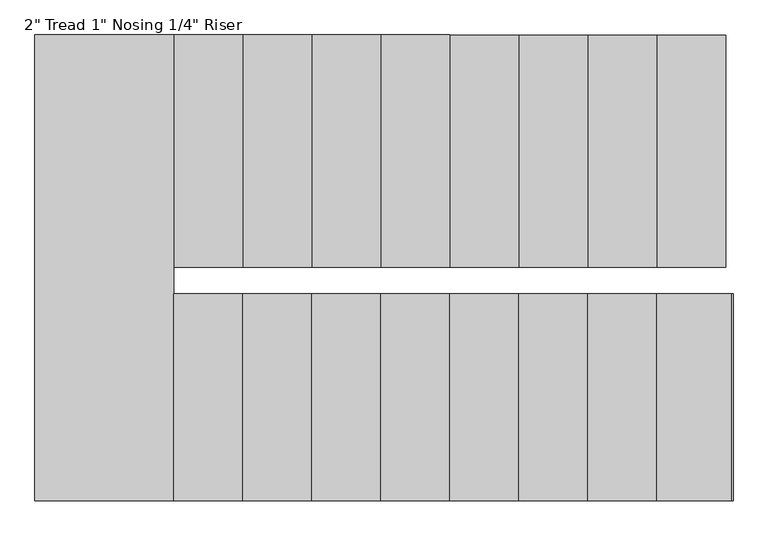
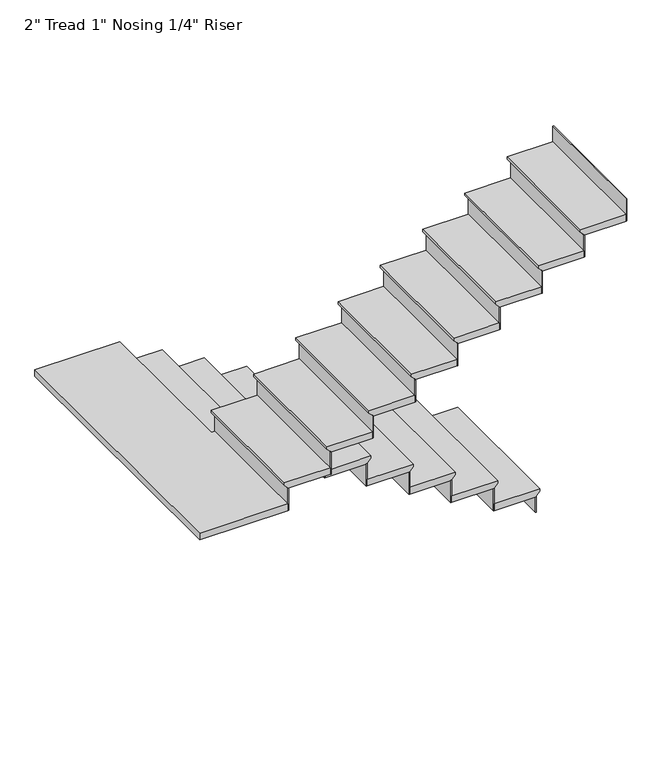
"""IFC4 building model written with IfcOpenShell, lengths in millimetres: stair flight geometry."""

from ifc_helpers import new_model, si_unit, origin, place, context, project, spatial, faceted_brep, source, transform, mapped, element, save


def stair_flight_289fc41f(model_context):
    return source(origin(), model_context, "Body", "Brep", [
        faceted_brep([(4295.1355783, 9969.5, 3198.2833333), (4295.1355783, 9969.5, 3217.3333333), (4295.1355783, 8944.6068332, 3217.3333333), (4295.1355783, 8944.6068332, 3198.2833333), (4269.7355783, 9969.5, 3172.8833333), (4269.7355783, 8944.6068332, 3172.8833333), (3964.9355783, 9969.5, 3217.3333333), (3964.9355783, 8944.6068332, 3217.3333333), (4269.7355783, 8944.6068332, 3166.5333333), (3964.9355783, 8944.6068332, 3166.5333333), (3964.9355783, 9969.5, 3166.5333333), (4269.7355783, 9969.5, 3166.5333333)], [[[0, 1, 2, 3]], [[4, 0, 3, 5]], [[2, 1, 6, 7]], [[8, 9, 10, 11]], [[2, 7, 9, 8, 5, 3]], [[8, 11, 4, 5]], [[6, 1, 0, 4, 11, 10]], [[7, 6, 10, 9]]]),
        faceted_brep([(4269.7355783, 9969.5, 3166.5333333), (4269.7355783, 9969.5, 3048.0), (4263.3855783, 9969.5, 3048.0), (4263.3855783, 9969.5, 3166.5333333), (4269.7355783, 8944.6068332, 3166.5333333), (4263.3855783, 8944.6068332, 3166.5333333), (4263.3855783, 8944.6068332, 3048.0), (4269.7355783, 8944.6068332, 3048.0)], [[[0, 1, 2, 3]], [[4, 5, 6, 7]], [[1, 0, 4, 7]], [[2, 1, 7, 6]], [[3, 2, 6, 5]], [[0, 3, 5, 4]]]),
        faceted_brep([(3964.9355783, 9969.5, 3335.8666667), (3964.9355783, 9969.5, 3166.5333333), (3958.5855783, 9969.5, 3166.5333333), (3958.5855783, 9969.5, 3335.8666667), (3964.9355783, 8944.6068332, 3335.8666667), (3958.5855783, 8944.6068332, 3335.8666667), (3958.5855783, 8944.6068332, 3166.5333333), (3964.9355783, 8944.6068332, 3166.5333333)], [[[0, 1, 2, 3]], [[4, 5, 6, 7]], [[1, 0, 4, 7]], [[2, 1, 7, 6]], [[3, 2, 6, 5]], [[0, 3, 5, 4]]]),
        faceted_brep([(3990.3355783, 8944.6068332, 3386.6666667), (3990.3355783, 9969.5, 3386.6666667), (3660.1355783, 9969.5, 3386.6666667), (3660.1355783, 8944.6068332, 3386.6666667), (3964.9355783, 8944.6068332, 3335.8666667), (3660.1355783, 8944.6068332, 3335.8666667), (3660.1355783, 9969.5, 3335.8666667), (3964.9355783, 9969.5, 3335.8666667), (3964.9355783, 8944.6068332, 3342.2166667), (3990.3355783, 8944.6068332, 3367.6166667), (3964.9355783, 9969.5, 3342.2166667), (3990.3355783, 9969.5, 3367.6166667)], [[[0, 1, 2, 3]], [[4, 5, 6, 7]], [[0, 3, 5, 4, 8, 9]], [[4, 7, 10, 8]], [[2, 1, 11, 10, 7, 6]], [[3, 2, 6, 5]], [[11, 1, 0, 9]], [[10, 11, 9, 8]]]),
        faceted_brep([(3660.1355783, 9969.5, 3505.2), (3660.1355783, 9969.5, 3335.8666667), (3653.7855783, 9969.5, 3335.8666667), (3653.7855783, 9969.5, 3505.2), (3660.1355783, 8944.6068332, 3505.2), (3653.7855783, 8944.6068332, 3505.2), (3653.7855783, 8944.6068332, 3335.8666667), (3660.1355783, 8944.6068332, 3335.8666667)], [[[0, 1, 2, 3]], [[4, 5, 6, 7]], [[1, 0, 4, 7]], [[2, 1, 7, 6]], [[3, 2, 6, 5]], [[0, 3, 5, 4]]]),
        faceted_brep([(3685.5355783, 8944.6068332, 3556.0), (3685.5355783, 9969.5, 3556.0), (3355.3355783, 9969.5, 3556.0), (3355.3355783, 8944.6068332, 3556.0), (3660.1355783, 8944.6068332, 3505.2), (3355.3355783, 8944.6068332, 3505.2), (3355.3355783, 9969.5, 3505.2), (3660.1355783, 9969.5, 3505.2), (3660.1355783, 8944.6068332, 3511.55), (3685.5355783, 8944.6068332, 3536.95), (3660.1355783, 9969.5, 3511.55), (3685.5355783, 9969.5, 3536.95)], [[[0, 1, 2, 3]], [[4, 5, 6, 7]], [[0, 3, 5, 4, 8, 9]], [[4, 7, 10, 8]], [[2, 1, 11, 10, 7, 6]], [[3, 2, 6, 5]], [[11, 1, 0, 9]], [[10, 11, 9, 8]]]),
        faceted_brep([(3355.3355783, 9969.5, 3674.5333333), (3355.3355783, 9969.5, 3505.2), (3348.9855783, 9969.5, 3505.2), (3348.9855783, 9969.5, 3674.5333333), (3355.3355783, 8944.6068332, 3674.5333333), (3348.9855783, 8944.6068332, 3674.5333333), (3348.9855783, 8944.6068332, 3505.2), (3355.3355783, 8944.6068332, 3505.2)], [[[0, 1, 2, 3]], [[4, 5, 6, 7]], [[1, 0, 4, 7]], [[2, 1, 7, 6]], [[3, 2, 6, 5]], [[0, 3, 5, 4]]]),
        faceted_brep([(3380.7355783, 8944.6068332, 3725.3333333), (3380.7355783, 9969.5, 3725.3333333), (3050.5355783, 9969.5, 3725.3333333), (3050.5355783, 8944.6068332, 3725.3333333), (3355.3355783, 8944.6068332, 3674.5333333), (3050.5355783, 8944.6068332, 3674.5333333), (3050.5355783, 9969.5, 3674.5333333), (3355.3355783, 9969.5, 3674.5333333), (3355.3355783, 8944.6068332, 3680.8833333), (3380.7355783, 8944.6068332, 3706.2833333), (3355.3355783, 9969.5, 3680.8833333), (3380.7355783, 9969.5, 3706.2833333)], [[[0, 1, 2, 3]], [[4, 5, 6, 7]], [[0, 3, 5, 4, 8, 9]], [[4, 7, 10, 8]], [[2, 1, 11, 10, 7, 6]], [[3, 2, 6, 5]], [[11, 1, 0, 9]], [[10, 11, 9, 8]]]),
        faceted_brep([(3050.5355783, 9969.5, 3843.8666667), (3050.5355783, 9969.5, 3674.5333333), (3044.1855783, 9969.5, 3674.5333333), (3044.1855783, 9969.5, 3843.8666667), (3050.5355783, 8944.6068332, 3843.8666667), (3044.1855783, 8944.6068332, 3843.8666667), (3044.1855783, 8944.6068332, 3674.5333333), (3050.5355783, 8944.6068332, 3674.5333333)], [[[0, 1, 2, 3]], [[4, 5, 6, 7]], [[1, 0, 4, 7]], [[2, 1, 7, 6]], [[3, 2, 6, 5]], [[0, 3, 5, 4]]]),
        faceted_brep([(3075.9355783, 8944.6068332, 3894.6666667), (3075.9355783, 9969.5, 3894.6666667), (2745.7355783, 9969.5, 3894.6666667), (2745.7355783, 8944.6068332, 3894.6666667), (3050.5355783, 8944.6068332, 3843.8666667), (2745.7355783, 8944.6068332, 3843.8666667), (2745.7355783, 9969.5, 3843.8666667), (3050.5355783, 9969.5, 3843.8666667), (3050.5355783, 8944.6068332, 3850.2166667), (3075.9355783, 8944.6068332, 3875.6166667), (3050.5355783, 9969.5, 3850.2166667), (3075.9355783, 9969.5, 3875.6166667)], [[[0, 1, 2, 3]], [[4, 5, 6, 7]], [[0, 3, 5, 4, 8, 9]], [[4, 7, 10, 8]], [[2, 1, 11, 10, 7, 6]], [[3, 2, 6, 5]], [[11, 1, 0, 9]], [[10, 11, 9, 8]]]),
        faceted_brep([(2745.7355783, 9969.5, 4013.2), (2745.7355783, 9969.5, 3843.8666667), (2739.3855783, 9969.5, 3843.8666667), (2739.3855783, 9969.5, 4013.2), (2745.7355783, 8944.6068332, 4013.2), (2739.3855783, 8944.6068332, 4013.2), (2739.3855783, 8944.6068332, 3843.8666667), (2745.7355783, 8944.6068332, 3843.8666667)], [[[0, 1, 2, 3]], [[4, 5, 6, 7]], [[1, 0, 4, 7]], [[2, 1, 7, 6]], [[3, 2, 6, 5]], [[0, 3, 5, 4]]]),
        faceted_brep([(2771.1355783, 8944.6068332, 4064.0), (2771.1355783, 9969.5, 4064.0), (2440.9355783, 9969.5, 4064.0), (2440.9355783, 8944.6068332, 4064.0), (2745.7355783, 8944.6068332, 4013.2), (2440.9355783, 8944.6068332, 4013.2), (2440.9355783, 9969.5, 4013.2), (2745.7355783, 9969.5, 4013.2), (2745.7355783, 8944.6068332, 4019.55), (2771.1355783, 8944.6068332, 4044.95), (2745.7355783, 9969.5, 4019.55), (2771.1355783, 9969.5, 4044.95)], [[[0, 1, 2, 3]], [[4, 5, 6, 7]], [[0, 3, 5, 4, 8, 9]], [[4, 7, 10, 8]], [[2, 1, 11, 10, 7, 6]], [[3, 2, 6, 5]], [[11, 1, 0, 9]], [[10, 11, 9, 8]]]),
        faceted_brep([(2440.9355783, 9969.5, 4182.5333333), (2440.9355783, 9969.5, 4013.2), (2434.5855783, 9969.5, 4013.2), (2434.5855783, 9969.5, 4182.5333333), (2440.9355783, 8944.6068332, 4182.5333333), (2434.5855783, 8944.6068332, 4182.5333333), (2434.5855783, 8944.6068332, 4013.2), (2440.9355783, 8944.6068332, 4013.2)], [[[0, 1, 2, 3]], [[4, 5, 6, 7]], [[1, 0, 4, 7]], [[2, 1, 7, 6]], [[3, 2, 6, 5]], [[0, 3, 5, 4]]]),
        faceted_brep([(2466.3355783, 8944.6068332, 4233.3333333), (2466.3355783, 9969.5, 4233.3333333), (2136.1355783, 9969.5, 4233.3333333), (2136.1355783, 8944.6068332, 4233.3333333), (2440.9355783, 8944.6068332, 4182.5333333), (2136.1355783, 8944.6068332, 4182.5333333), (2136.1355783, 9969.5, 4182.5333333), (2440.9355783, 9969.5, 4182.5333333), (2440.9355783, 8944.6068332, 4188.8833333), (2466.3355783, 8944.6068332, 4214.2833333), (2440.9355783, 9969.5, 4188.8833333), (2466.3355783, 9969.5, 4214.2833333)], [[[0, 1, 2, 3]], [[4, 5, 6, 7]], [[0, 3, 5, 4, 8, 9]], [[4, 7, 10, 8]], [[2, 1, 11, 10, 7, 6]], [[3, 2, 6, 5]], [[11, 1, 0, 9]], [[10, 11, 9, 8]]]),
        faceted_brep([(2136.1355783, 9969.5, 4351.8666667), (2136.1355783, 9969.5, 4182.5333333), (2129.7855783, 9969.5, 4182.5333333), (2129.7855783, 9969.5, 4351.8666667), (2136.1355783, 8944.6068332, 4351.8666667), (2129.7855783, 8944.6068332, 4351.8666667), (2129.7855783, 8944.6068332, 4182.5333333), (2136.1355783, 8944.6068332, 4182.5333333)], [[[0, 1, 2, 3]], [[4, 5, 6, 7]], [[1, 0, 4, 7]], [[2, 1, 7, 6]], [[3, 2, 6, 5]], [[0, 3, 5, 4]]]),
        faceted_brep([(2161.5355783, 8944.6068332, 4402.6666667), (2161.5355783, 9969.5, 4402.6666667), (1831.3355783, 9969.5, 4402.6666667), (1831.3355783, 8944.6068332, 4402.6666667), (2136.1355783, 8944.6068332, 4351.8666667), (1831.3355783, 8944.6068332, 4351.8666667), (1831.3355783, 9969.5, 4351.8666667), (2136.1355783, 9969.5, 4351.8666667), (2136.1355783, 8944.6068332, 4358.2166667), (2161.5355783, 8944.6068332, 4383.6166667), (2136.1355783, 9969.5, 4358.2166667), (2161.5355783, 9969.5, 4383.6166667)], [[[0, 1, 2, 3]], [[4, 5, 6, 7]], [[0, 3, 5, 4, 8, 9]], [[4, 7, 10, 8]], [[2, 1, 11, 10, 7, 6]], [[3, 2, 6, 5]], [[11, 1, 0, 9]], [[10, 11, 9, 8]]]),
        faceted_brep([(1831.3355783, 9969.5, 4521.2), (1831.3355783, 9969.5, 4351.8666667), (1824.9855783, 9969.5, 4351.8666667), (1824.9855783, 9969.5, 4521.2), (1831.3355783, 8944.6068332, 4521.2), (1824.9855783, 8944.6068332, 4521.2), (1824.9855783, 8944.6068332, 4351.8666667), (1831.3355783, 8944.6068332, 4351.8666667)], [[[0, 1, 2, 3]], [[4, 5, 6, 7]], [[1, 0, 4, 7]], [[2, 1, 7, 6]], [[3, 2, 6, 5]], [[0, 3, 5, 4]]]),
        faceted_brep([(1882.1355783, 8826.5, 4572.0), (1856.7355783, 8826.5, 4572.0), (1856.7355783, 9969.5, 4572.0), (1244.6, 9969.5, 4572.0), (1244.6, 7912.1, 4572.0), (1882.1355783, 7912.1, 4572.0), (1856.7355783, 8826.5, 4521.2), (1882.1355783, 8826.5, 4521.2), (1882.1355783, 7912.1, 4521.2), (1244.6, 7912.1, 4521.2), (1244.6, 9969.5, 4521.2), (1831.3355783, 9969.5, 4521.2), (1831.3355783, 8944.6068332, 4521.2), (1856.7355783, 8944.6068332, 4521.2), (1856.7355783, 8944.6068332, 4552.95), (1856.7355783, 9969.5, 4552.95), (1831.3355783, 8944.6068332, 4527.55), (1831.3355783, 9969.5, 4527.55)], [[[0, 1, 2, 3, 4, 5]], [[6, 7, 8, 9, 10, 11, 12, 13]], [[1, 0, 7, 6]], [[2, 1, 6, 13, 14, 15]], [[13, 12, 16, 14]], [[12, 11, 17, 16]], [[3, 2, 15, 17, 11, 10]], [[4, 3, 10, 9]], [[5, 4, 9, 8]], [[0, 5, 8, 7]], [[17, 15, 14, 16]]]),
        faceted_brep([(1882.1355783, 7912.1, 4690.5333333), (1882.1355783, 7912.1, 4521.2), (1888.4855783, 7912.1, 4521.2), (1888.4855783, 7912.1, 4690.5333333), (1882.1355783, 8826.5, 4690.5333333), (1888.4855783, 8826.5, 4690.5333333), (1888.4855783, 8826.5, 4521.2), (1882.1355783, 8826.5, 4521.2)], [[[0, 1, 2, 3]], [[4, 5, 6, 7]], [[1, 0, 4, 7]], [[2, 1, 7, 6]], [[3, 2, 6, 5]], [[0, 3, 5, 4]]]),
        faceted_brep([(1856.7355783, 8826.5, 4741.3333333), (1856.7355783, 7912.1, 4741.3333333), (2186.9355783, 7912.1, 4741.3333333), (2186.9355783, 8826.5, 4741.3333333), (1882.1355783, 8826.5, 4690.5333333), (2186.9355783, 8826.5, 4690.5333333), (2186.9355783, 7912.1, 4690.5333333), (1882.1355783, 7912.1, 4690.5333333), (1882.1355783, 8826.5, 4696.8833333), (1856.7355783, 8826.5, 4722.2833333), (1882.1355783, 7912.1, 4696.8833333), (1856.7355783, 7912.1, 4722.2833333)], [[[0, 1, 2, 3]], [[4, 5, 6, 7]], [[0, 3, 5, 4, 8, 9]], [[4, 7, 10, 8]], [[2, 1, 11, 10, 7, 6]], [[3, 2, 6, 5]], [[11, 1, 0, 9]], [[10, 11, 9, 8]]]),
        faceted_brep([(2186.9355783, 7912.1, 4859.8666667), (2186.9355783, 7912.1, 4690.5333333), (2193.2855783, 7912.1, 4690.5333333), (2193.2855783, 7912.1, 4859.8666667), (2186.9355783, 8826.5, 4859.8666667), (2193.2855783, 8826.5, 4859.8666667), (2193.2855783, 8826.5, 4690.5333333), (2186.9355783, 8826.5, 4690.5333333)], [[[0, 1, 2, 3]], [[4, 5, 6, 7]], [[1, 0, 4, 7]], [[2, 1, 7, 6]], [[3, 2, 6, 5]], [[0, 3, 5, 4]]]),
        faceted_brep([(2161.5355783, 8826.5, 4910.6666667), (2161.5355783, 7912.1, 4910.6666667), (2491.7355783, 7912.1, 4910.6666667), (2491.7355783, 8826.5, 4910.6666667), (2186.9355783, 8826.5, 4859.8666667), (2491.7355783, 8826.5, 4859.8666667), (2491.7355783, 7912.1, 4859.8666667), (2186.9355783, 7912.1, 4859.8666667), (2186.9355783, 8826.5, 4866.2166667), (2161.5355783, 8826.5, 4891.6166667), (2186.9355783, 7912.1, 4866.2166667), (2161.5355783, 7912.1, 4891.6166667)], [[[0, 1, 2, 3]], [[4, 5, 6, 7]], [[0, 3, 5, 4, 8, 9]], [[4, 7, 10, 8]], [[2, 1, 11, 10, 7, 6]], [[3, 2, 6, 5]], [[11, 1, 0, 9]], [[10, 11, 9, 8]]]),
        faceted_brep([(2491.7355783, 7912.1, 5029.2), (2491.7355783, 7912.1, 4859.8666667), (2498.0855783, 7912.1, 4859.8666667), (2498.0855783, 7912.1, 5029.2), (2491.7355783, 8826.5, 5029.2), (2498.0855783, 8826.5, 5029.2), (2498.0855783, 8826.5, 4859.8666667), (2491.7355783, 8826.5, 4859.8666667)], [[[0, 1, 2, 3]], [[4, 5, 6, 7]], [[1, 0, 4, 7]], [[2, 1, 7, 6]], [[3, 2, 6, 5]], [[0, 3, 5, 4]]]),
        faceted_brep([(2466.3355783, 8826.5, 5080.0), (2466.3355783, 7912.1, 5080.0), (2796.5355783, 7912.1, 5080.0), (2796.5355783, 8826.5, 5080.0), (2491.7355783, 8826.5, 5029.2), (2796.5355783, 8826.5, 5029.2), (2796.5355783, 7912.1, 5029.2), (2491.7355783, 7912.1, 5029.2), (2491.7355783, 8826.5, 5035.55), (2466.3355783, 8826.5, 5060.95), (2491.7355783, 7912.1, 5035.55), (2466.3355783, 7912.1, 5060.95)], [[[0, 1, 2, 3]], [[4, 5, 6, 7]], [[0, 3, 5, 4, 8, 9]], [[4, 7, 10, 8]], [[2, 1, 11, 10, 7, 6]], [[3, 2, 6, 5]], [[11, 1, 0, 9]], [[10, 11, 9, 8]]]),
        faceted_brep([(2796.5355783, 7912.1, 5198.5333333), (2796.5355783, 7912.1, 5029.2), (2802.8855783, 7912.1, 5029.2), (2802.8855783, 7912.1, 5198.5333333), (2796.5355783, 8826.5, 5198.5333333), (2802.8855783, 8826.5, 5198.5333333), (2802.8855783, 8826.5, 5029.2), (2796.5355783, 8826.5, 5029.2)], [[[0, 1, 2, 3]], [[4, 5, 6, 7]], [[1, 0, 4, 7]], [[2, 1, 7, 6]], [[3, 2, 6, 5]], [[0, 3, 5, 4]]]),
        faceted_brep([(2771.1355783, 8826.5, 5249.3333333), (2771.1355783, 7912.1, 5249.3333333), (3101.3355783, 7912.1, 5249.3333333), (3101.3355783, 8826.5, 5249.3333333), (2796.5355783, 8826.5, 5198.5333333), (3101.3355783, 8826.5, 5198.5333333), (3101.3355783, 7912.1, 5198.5333333), (2796.5355783, 7912.1, 5198.5333333), (2796.5355783, 8826.5, 5204.8833333), (2771.1355783, 8826.5, 5230.2833333), (2796.5355783, 7912.1, 5204.8833333), (2771.1355783, 7912.1, 5230.2833333)], [[[0, 1, 2, 3]], [[4, 5, 6, 7]], [[0, 3, 5, 4, 8, 9]], [[4, 7, 10, 8]], [[2, 1, 11, 10, 7, 6]], [[3, 2, 6, 5]], [[11, 1, 0, 9]], [[10, 11, 9, 8]]]),
        faceted_brep([(3101.3355783, 7912.1, 5367.8666667), (3101.3355783, 7912.1, 5198.5333333), (3107.6855783, 7912.1, 5198.5333333), (3107.6855783, 7912.1, 5367.8666667), (3101.3355783, 8826.5, 5367.8666667), (3107.6855783, 8826.5, 5367.8666667), (3107.6855783, 8826.5, 5198.5333333), (3101.3355783, 8826.5, 5198.5333333)], [[[0, 1, 2, 3]], [[4, 5, 6, 7]], [[1, 0, 4, 7]], [[2, 1, 7, 6]], [[3, 2, 6, 5]], [[0, 3, 5, 4]]]),
        faceted_brep([(3075.9355783, 8826.5, 5418.6666667), (3075.9355783, 7912.1, 5418.6666667), (3406.1355783, 7912.1, 5418.6666667), (3406.1355783, 8826.5, 5418.6666667), (3101.3355783, 8826.5, 5367.8666667), (3406.1355783, 8826.5, 5367.8666667), (3406.1355783, 7912.1, 5367.8666667), (3101.3355783, 7912.1, 5367.8666667), (3101.3355783, 8826.5, 5374.2166667), (3075.9355783, 8826.5, 5399.6166667), (3101.3355783, 7912.1, 5374.2166667), (3075.9355783, 7912.1, 5399.6166667)], [[[0, 1, 2, 3]], [[4, 5, 6, 7]], [[0, 3, 5, 4, 8, 9]], [[4, 7, 10, 8]], [[2, 1, 11, 10, 7, 6]], [[3, 2, 6, 5]], [[11, 1, 0, 9]], [[10, 11, 9, 8]]]),
        faceted_brep([(3406.1355783, 7912.1, 5537.2), (3406.1355783, 7912.1, 5367.8666667), (3412.4855783, 7912.1, 5367.8666667), (3412.4855783, 7912.1, 5537.2), (3406.1355783, 8826.5, 5537.2), (3412.4855783, 8826.5, 5537.2), (3412.4855783, 8826.5, 5367.8666667), (3406.1355783, 8826.5, 5367.8666667)], [[[0, 1, 2, 3]], [[4, 5, 6, 7]], [[1, 0, 4, 7]], [[2, 1, 7, 6]], [[3, 2, 6, 5]], [[0, 3, 5, 4]]]),
        faceted_brep([(3380.7355783, 8826.5, 5588.0), (3380.7355783, 7912.1, 5588.0), (3710.9355783, 7912.1, 5588.0), (3710.9355783, 8826.5, 5588.0), (3406.1355783, 8826.5, 5537.2), (3710.9355783, 8826.5, 5537.2), (3710.9355783, 7912.1, 5537.2), (3406.1355783, 7912.1, 5537.2), (3406.1355783, 8826.5, 5543.55), (3380.7355783, 8826.5, 5568.95), (3406.1355783, 7912.1, 5543.55), (3380.7355783, 7912.1, 5568.95)], [[[0, 1, 2, 3]], [[4, 5, 6, 7]], [[0, 3, 5, 4, 8, 9]], [[4, 7, 10, 8]], [[2, 1, 11, 10, 7, 6]], [[3, 2, 6, 5]], [[11, 1, 0, 9]], [[10, 11, 9, 8]]]),
        faceted_brep([(3710.9355783, 7912.1, 5706.5333333), (3710.9355783, 7912.1, 5537.2), (3717.2855783, 7912.1, 5537.2), (3717.2855783, 7912.1, 5706.5333333), (3710.9355783, 8826.5, 5706.5333333), (3717.2855783, 8826.5, 5706.5333333), (3717.2855783, 8826.5, 5537.2), (3710.9355783, 8826.5, 5537.2)], [[[0, 1, 2, 3]], [[4, 5, 6, 7]], [[1, 0, 4, 7]], [[2, 1, 7, 6]], [[3, 2, 6, 5]], [[0, 3, 5, 4]]]),
        faceted_brep([(3685.5355783, 8826.5, 5757.3333333), (3685.5355783, 7912.1, 5757.3333333), (4015.7355783, 7912.1, 5757.3333333), (4015.7355783, 8826.5, 5757.3333333), (3710.9355783, 8826.5, 5706.5333333), (4015.7355783, 8826.5, 5706.5333333), (4015.7355783, 7912.1, 5706.5333333), (3710.9355783, 7912.1, 5706.5333333), (3710.9355783, 8826.5, 5712.8833333), (3685.5355783, 8826.5, 5738.2833333), (3710.9355783, 7912.1, 5712.8833333), (3685.5355783, 7912.1, 5738.2833333)], [[[0, 1, 2, 3]], [[4, 5, 6, 7]], [[0, 3, 5, 4, 8, 9]], [[4, 7, 10, 8]], [[2, 1, 11, 10, 7, 6]], [[3, 2, 6, 5]], [[11, 1, 0, 9]], [[10, 11, 9, 8]]]),
        faceted_brep([(4015.7355783, 7912.1, 5875.8666667), (4015.7355783, 7912.1, 5706.5333333), (4022.0855783, 7912.1, 5706.5333333), (4022.0855783, 7912.1, 5875.8666667), (4015.7355783, 8826.5, 5875.8666667), (4022.0855783, 8826.5, 5875.8666667), (4022.0855783, 8826.5, 5706.5333333), (4015.7355783, 8826.5, 5706.5333333)], [[[0, 1, 2, 3]], [[4, 5, 6, 7]], [[1, 0, 4, 7]], [[2, 1, 7, 6]], [[3, 2, 6, 5]], [[0, 3, 5, 4]]]),
        faceted_brep([(4320.5355783, 7912.1, 6045.2), (4320.5355783, 7912.1, 5875.8666667), (4326.8855783, 7912.1, 5875.8666667), (4326.8855783, 7912.1, 6045.2), (4320.5355783, 8826.5, 6045.2), (4326.8855783, 8826.5, 6045.2), (4326.8855783, 8826.5, 5875.8666667), (4320.5355783, 8826.5, 5875.8666667)], [[[0, 1, 2, 3]], [[4, 5, 6, 7]], [[1, 0, 4, 7]], [[2, 1, 7, 6]], [[3, 2, 6, 5]], [[0, 3, 5, 4]]]),
        faceted_brep([(3990.3355783, 8826.5, 5926.6666667), (3990.3355783, 7912.1, 5926.6666667), (4320.5355783, 7912.1, 5926.6666667), (4320.5355783, 8826.5, 5926.6666667), (4015.7355783, 8826.5, 5875.8666667), (4320.5355783, 8826.5, 5875.8666667), (4320.5355783, 7912.1, 5875.8666667), (4015.7355783, 7912.1, 5875.8666667), (4015.7355783, 8826.5, 5882.2166667), (3990.3355783, 8826.5, 5907.6166667), (4015.7355783, 7912.1, 5882.2166667), (3990.3355783, 7912.1, 5907.6166667)], [[[0, 1, 2, 3]], [[4, 5, 6, 7]], [[0, 3, 5, 4, 8, 9]], [[4, 7, 10, 8]], [[2, 1, 11, 10, 7, 6]], [[3, 2, 6, 5]], [[11, 1, 0, 9]], [[10, 11, 9, 8]]]),
    ])


if __name__ == "__main__":
    model = new_model("IFC4")
    model_context = context("Model", 3, world=origin())
    ifc_project = project(units=[si_unit("LENGTHUNIT", "METRE", prefix="MILLI")], contexts=[model_context])
    site = spatial("IfcSite", under=ifc_project)
    building = spatial("IfcBuilding", under=site)
    placement = place(None, origin())
    stair_flight_shape = stair_flight_289fc41f(model_context)
    element("IfcStairFlight", 1, ObjectType="2\" Tread 1\" Nosing 1/4\" Riser", at=placement, inside=building, context=model_context, shape_type="MappedRepresentation", body=[
        mapped(stair_flight_shape, transform((0.0, 0.0, 0.0), x_axis=(1.0, 0.0, 0.0), y_axis=(0.0, 1.0, 0.0), z_axis=(0.0, 0.0, 1.0))),
    ])
    save(model, "model.ifc")
